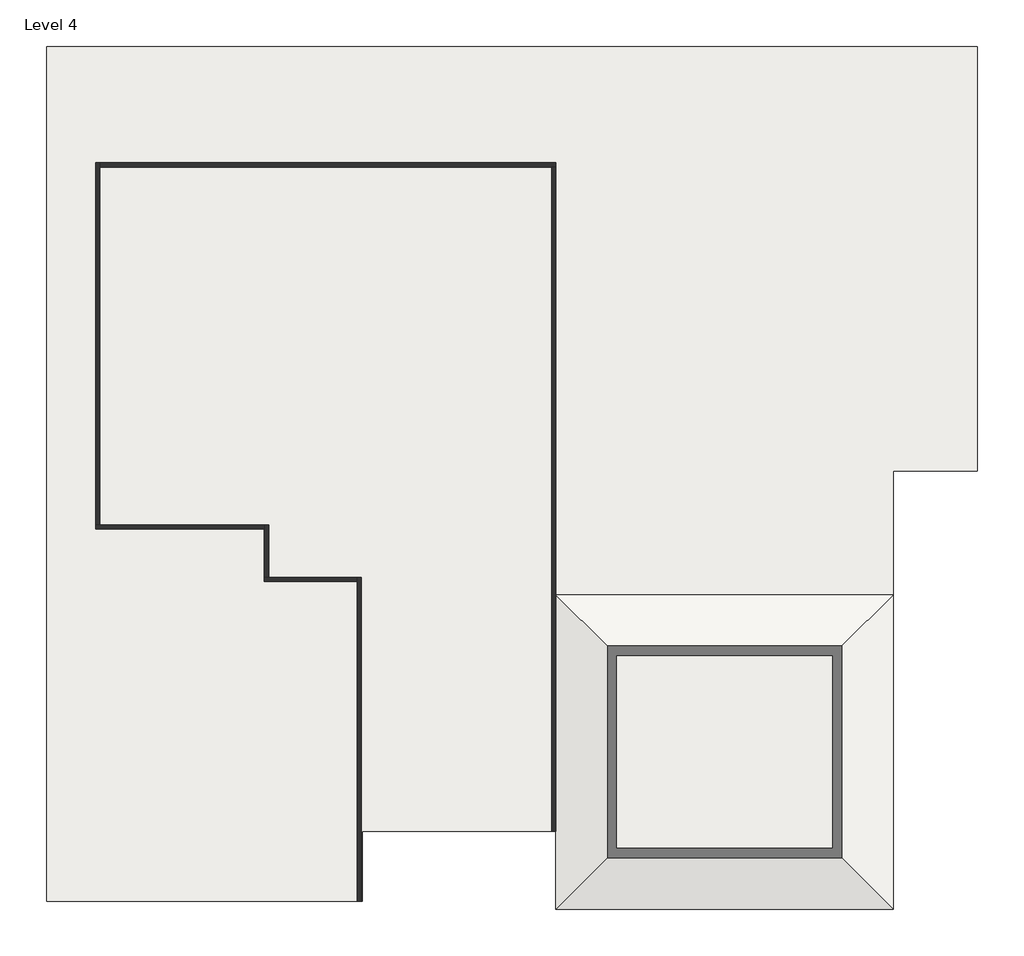
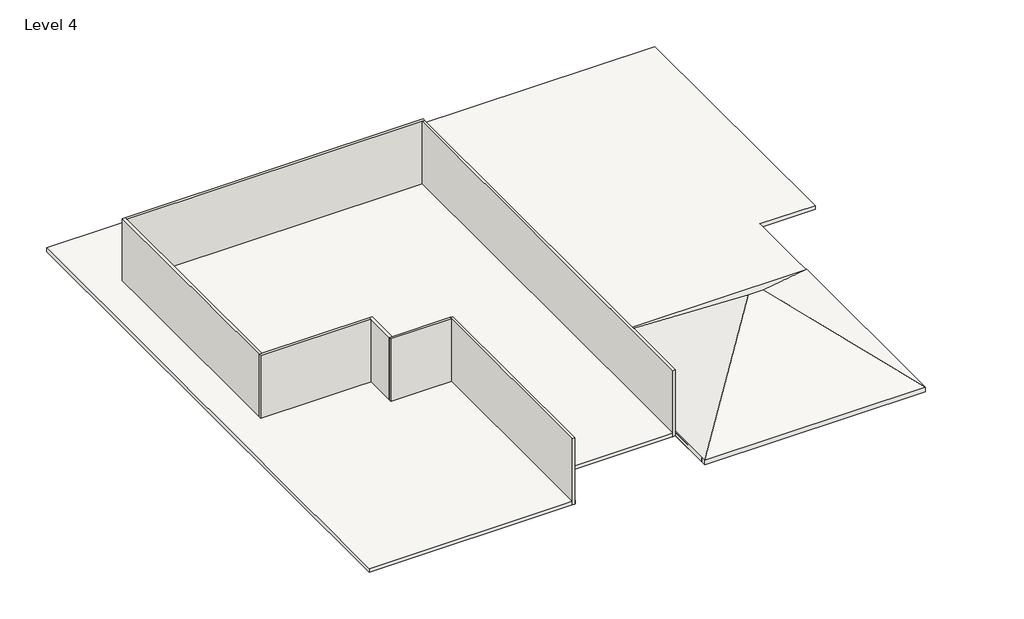
# One storey, incomplete: 7 walls, 2 roofs.
"""IFC4 building model written with IfcOpenShell, lengths in millimetres."""

from ifc_helpers import new_model, si_unit, frame, origin, place, context, project, spatial, polyline, outline, extrude, faceted_brep, element, save

model = new_model("IFC4")

# Units and contexts
model_context = context("Model", 3, world=origin())
ifc_project = project(units=[si_unit("LENGTHUNIT", "METRE", prefix="MILLI")], contexts=[model_context])

# Site, building, storey
site = spatial("IfcSite", under=ifc_project)
building = spatial("IfcBuilding", under=site)
storey = spatial("IfcBuildingStorey", under=building, Name="Level 4", Elevation=8432.8)

# Roofs
placement = place(None, origin())
element("IfcRoof", 1, ObjectType="6\"", at=placement, inside=storey, context=model_context, shape_type="SweptSolid", body=[
    extrude(outline(polyline([(-15479.9059085, 17481.4414483), (8904.0940915, 17481.4414483), (8904.0940915, 6356.2414483), (6694.2940915, 6356.2414483), (6694.2940915, -4921.3585517), (-2144.9059085, -4921.3585517), (-2144.9059085, -3092.5585517), (-7212.2059085, -3092.5585517), (-7212.2059085, -4921.3585517), (-15479.9059085, -4921.3585517), (-15479.9059085, 17481.4414483)])), frame((0.0, 0.0, 8432.8), z_axis=(0.0, 0.0, 1.0), x_axis=(1.0, 0.0, 0.0)), (0.0, 0.0, 1.0), 152.4),
])
element("IfcRoof", 2, ObjectType="6\" 2", at=placement, inside=storey, context=model_context, shape_type="Brep", body=[
    faceted_brep([(-2144.9059085, -5124.5585517, 8432.8), (1974.1480602, -1005.5045831, 11522.0904765), (2575.2401228, -1005.5045831, 11522.0904765), (6694.2940915, -5124.5585517, 8432.8), (6694.2940915, 3113.5493856, 8432.8), (-2144.9059085, 3113.5493856, 8432.8), (-2144.9059085, -5124.5585517, 8623.3), (6694.2940915, -5124.5585517, 8623.3), (2575.2401228, -1005.5045831, 11712.5904765), (1974.1480602, -1005.5045831, 11712.5904765), (6694.2940915, 3113.5493856, 8623.3), (-2144.9059085, 3113.5493856, 8623.3)], [[[0, 1, 2, 3]], [[3, 2, 4]], [[4, 2, 1, 5]], [[1, 0, 5]], [[6, 7, 8, 9]], [[7, 10, 8]], [[10, 11, 9, 8]], [[6, 9, 11]], [[3, 7, 6, 0]], [[4, 10, 7, 3]], [[5, 11, 10, 4]], [[0, 6, 11, 5]]]),
])

# Walls
element("IfcWall", 3, ObjectType="4\"", at=placement, inside=storey, context=model_context, shape_type="Brep", body=[
    faceted_brep([(-7237.6059085, 3562.2414483, 11233.15), (-7237.6059085, -4921.3585517, 11233.15), (-7237.6059085, -4921.3585517, 8432.8), (-7237.6059085, -3092.5585517, 8432.8), (-7237.6059085, -3092.5585517, 8483.6), (-7237.6059085, -2863.9585517, 8483.6), (-7237.6059085, -2863.9585517, 8432.8), (-7237.6059085, 1936.6414483, 8432.8), (-7237.6059085, 1936.6414483, 8483.6), (-7237.6059085, 2165.2414483, 8483.6), (-7237.6059085, 2165.2414483, 8432.8), (-7237.6059085, 3562.2414483, 8432.8), (-7339.2059085, -4921.3585517, 11233.15), (-7339.2059085, 3460.6414483, 11233.15), (-7339.2059085, 3562.2414483, 11233.15), (-7339.2059085, 3562.2414483, 8432.8), (-7339.2059085, 3460.6414483, 8432.8), (-7339.2059085, 2165.2414483, 8432.8), (-7339.2059085, 2165.2414483, 8483.6), (-7339.2059085, 1936.6414483, 8483.6), (-7339.2059085, 1936.6414483, 8432.8), (-7339.2059085, -2863.9585517, 8432.8), (-7339.2059085, -2863.9585517, 8483.6), (-7339.2059085, -3092.5585517, 8483.6), (-7339.2059085, -3092.5585517, 8432.8), (-7339.2059085, -4921.3585517, 8432.8)], [[[0, 1, 2, 3, 4, 5, 6, 7, 8, 9, 10, 11]], [[12, 13, 14, 15, 16, 17, 18, 19, 20, 21, 22, 23, 24, 25]], [[2, 25, 24, 3]], [[11, 10, 17, 16, 15]], [[20, 7, 6, 21]], [[1, 0, 14, 13, 12]], [[2, 1, 12, 25]], [[9, 18, 17, 10]], [[19, 8, 7, 20]], [[18, 9, 8, 19]], [[5, 22, 21, 6]], [[23, 4, 3, 24]], [[22, 5, 4, 23]], [[0, 11, 15, 14]]]),
])
element("IfcWall", 4, ObjectType="4\"", at=placement, inside=storey, context=model_context, shape_type="Brep", body=[
    faceted_brep([(-7339.2059085, 3562.2414483, 8432.8), (-9663.3059085, 3562.2414483, 8432.8), (-9777.6059085, 3562.2414483, 8432.8), (-9777.6059085, 3562.2414483, 11233.15), (-9663.3059085, 3562.2414483, 11233.15), (-7339.2059085, 3562.2414483, 11233.15), (-7339.2059085, 3460.6414483, 8432.8), (-7339.2059085, 3460.6414483, 11233.15), (-9777.6059085, 3460.6414483, 11233.15), (-9777.6059085, 3460.6414483, 8432.8)], [[[0, 1, 2, 3, 4, 5]], [[6, 7, 8, 9]], [[2, 1, 0, 6, 9]], [[5, 4, 3, 8, 7]], [[0, 5, 7, 6]], [[3, 2, 9, 8]]]),
])
element("IfcWall", 5, ObjectType="4\"", at=placement, inside=storey, context=model_context, shape_type="SweptSolid", body=[
    extrude(outline(polyline([(-2246.5059085, -3092.5585517), (-2246.5059085, 14319.1414483), (-2144.9059085, 14319.1414483), (-2144.9059085, -3092.5585517), (-2246.5059085, -3092.5585517)])), frame((0.0, 0.0, 8432.8), z_axis=(0.0, 0.0, 1.0), x_axis=(1.0, 0.0, 0.0)), (0.0, 0.0, 1.0), 2800.35),
])
element("IfcWall", 6, ObjectType="4.5\" wall", at=placement, inside=storey, context=model_context, shape_type="Brep", body=[
    faceted_brep([(-9663.3059085, 3562.2414483, 8432.8), (-9663.3059085, 4946.5414483, 8432.8), (-9663.3059085, 4946.5414483, 11233.15), (-9663.3059085, 3562.2414483, 11233.15), (-9777.6059085, 3562.2414483, 8432.8), (-9777.6059085, 3562.2414483, 11233.15), (-9777.6059085, 4832.2414483, 11233.15), (-9777.6059085, 4946.5414483, 11233.15), (-9777.6059085, 4946.5414483, 8432.8), (-9777.6059085, 4832.2414483, 8432.8)], [[[0, 1, 2, 3]], [[4, 5, 6, 7, 8, 9]], [[1, 0, 4, 9, 8]], [[3, 2, 7, 6, 5]], [[0, 3, 5, 4]], [[2, 1, 8, 7]]]),
])
element("IfcWall", 7, ObjectType="4.5\" wall", at=placement, inside=storey, context=model_context, shape_type="Brep", body=[
    faceted_brep([(-14197.2059085, 4946.5414483, 11233.15), (-14082.9059085, 4946.5414483, 11233.15), (-9777.6059085, 4946.5414483, 11233.15), (-9777.6059085, 4946.5414483, 8432.8), (-13422.5059085, 4946.5414483, 8432.8), (-13422.5059085, 4946.5414483, 8483.6), (-13651.1059085, 4946.5414483, 8483.6), (-13651.1059085, 4946.5414483, 8432.8), (-14082.9059085, 4946.5414483, 8432.8), (-14197.2059085, 4946.5414483, 8432.8), (-9777.6059085, 4832.2414483, 11233.15), (-14197.2059085, 4832.2414483, 11233.15), (-14197.2059085, 4832.2414483, 8432.8), (-13651.1059085, 4832.2414483, 8432.8), (-13651.1059085, 4832.2414483, 8483.6), (-13422.5059085, 4832.2414483, 8483.6), (-13422.5059085, 4832.2414483, 8432.8), (-9777.6059085, 4832.2414483, 8432.8)], [[[0, 1, 2, 3, 4, 5, 6, 7, 8, 9]], [[10, 11, 12, 13, 14, 15, 16, 17]], [[3, 17, 16, 4]], [[12, 9, 8, 7, 13]], [[2, 1, 0, 11, 10]], [[3, 2, 10, 17]], [[6, 14, 13, 7]], [[15, 5, 4, 16]], [[14, 6, 5, 15]], [[0, 9, 12, 11]]]),
])
element("IfcWall", 8, ObjectType="4.5\" wall", at=placement, inside=storey, context=model_context, shape_type="Brep", body=[
    faceted_brep([(-14082.9059085, 4946.5414483, 8432.8), (-14082.9059085, 14319.1414483, 8432.8), (-14082.9059085, 14433.4414483, 8432.8), (-14082.9059085, 14433.4414483, 11233.15), (-14082.9059085, 14319.1414483, 11233.15), (-14082.9059085, 4946.5414483, 11233.15), (-14197.2059085, 4946.5414483, 8432.8), (-14197.2059085, 4946.5414483, 11233.15), (-14197.2059085, 14433.4414483, 11233.15), (-14197.2059085, 14433.4414483, 8432.8)], [[[0, 1, 2, 3, 4, 5]], [[6, 7, 8, 9]], [[2, 1, 0, 6, 9]], [[5, 4, 3, 8, 7]], [[0, 5, 7, 6]], [[3, 2, 9, 8]]]),
])
element("IfcWall", 9, ObjectType="4.5\" wall", at=placement, inside=storey, context=model_context, shape_type="Brep", body=[
    faceted_brep([(-2144.9059085, 14319.1414483, 11233.15), (-2246.5059085, 14319.1414483, 11233.15), (-14082.9059085, 14319.1414483, 11233.15), (-14082.9059085, 14319.1414483, 8432.8), (-13651.1059085, 14319.1414483, 8432.8), (-13651.1059085, 14319.1414483, 8483.6), (-13422.5059085, 14319.1414483, 8483.6), (-13422.5059085, 14319.1414483, 8432.8), (-2246.5059085, 14319.1414483, 8432.8), (-2144.9059085, 14319.1414483, 8432.8), (-14082.9059085, 14433.4414483, 11233.15), (-2144.9059085, 14433.4414483, 11233.15), (-2144.9059085, 14433.4414483, 8432.8), (-13422.5059085, 14433.4414483, 8432.8), (-13422.5059085, 14433.4414483, 8483.6), (-13651.1059085, 14433.4414483, 8483.6), (-13651.1059085, 14433.4414483, 8432.8), (-14082.9059085, 14433.4414483, 8432.8)], [[[0, 1, 2, 3, 4, 5, 6, 7, 8, 9]], [[10, 11, 12, 13, 14, 15, 16, 17]], [[3, 17, 16, 4]], [[12, 9, 8, 7, 13]], [[2, 1, 0, 11, 10]], [[3, 2, 10, 17]], [[15, 5, 4, 16]], [[6, 14, 13, 7]], [[5, 15, 14, 6]], [[0, 9, 12, 11]]]),
])

save(model, "model.ifc")

# Revit data of these elements
# Type "6\""
#   Assembly Code = "B1020"
#   Layers, outside or top first: 0' - 6" "warm colour" (function 1)
# Type "6\" 2"
#   Assembly Code = "B1020"
#   Layers, outside or top first: 0' - 6" "roof" (function 1)
# Type "4\""
#   Assembly Code = "B2010"
#   Layers, outside or top first: 0' - 4" "ash colour window" (function 1)
# Type "4.5\" wall"
#   Assembly Code = "B2010"
#   Layers, outside or top first: 0' - 4 1/2" "ash colour window" (function 1)
# Element 1 (IfcRoof, "6\"")
#   built-in parameter 1001705 = 28.1667 (stored number, unit not read)
#   built-in parameter 1001701 = 0 (stored number, unit not read)
#   built-in parameter 1001710 = 33615
#   Phase Created = New Construction
#   Materials on its faces: "warm colour"
# Element 2 (IfcRoof, "6\" 2")
#   built-in parameter 1001705 = 38.4271 (stored number, unit not read)
#   built-in parameter 1001710 = 33615
#   Phase Created = New Construction
#   Materials on its faces: "roof"
# Elements 3, 4, 5 (IfcWall, "4\"")
#   Top Offset = 0' - 0"
#   Base Offset = 0' - 0"
#   wall height = 9' - 2 1/4"
#   Phase Created = New Construction
#   Base Constraint = Level 4
#   Top Constraint = Level 6
#   Materials on its faces: "ash colour window"
# Elements 6, 7, 8, 9 (IfcWall, "4.5\" wall")
#   Top Offset = 0' - 0"
#   Base Offset = 0' - 0"
#   wall height = 9' - 2 1/4"
#   Phase Created = New Construction
#   Base Constraint = Level 4
#   Top Constraint = Level 6
#   Materials on its faces: "ash colour window"
# Materials
#   "warm colour": class "Generic", colour RGB 120 120 120, transparency 0, Cost = 0
#   "roof": class "Generic", colour RGB 120 120 120, transparency 0, Cost = 0
#   "ash colour window": class "Generic", colour RGB 120 120 120, transparency 0, Cost = 0
